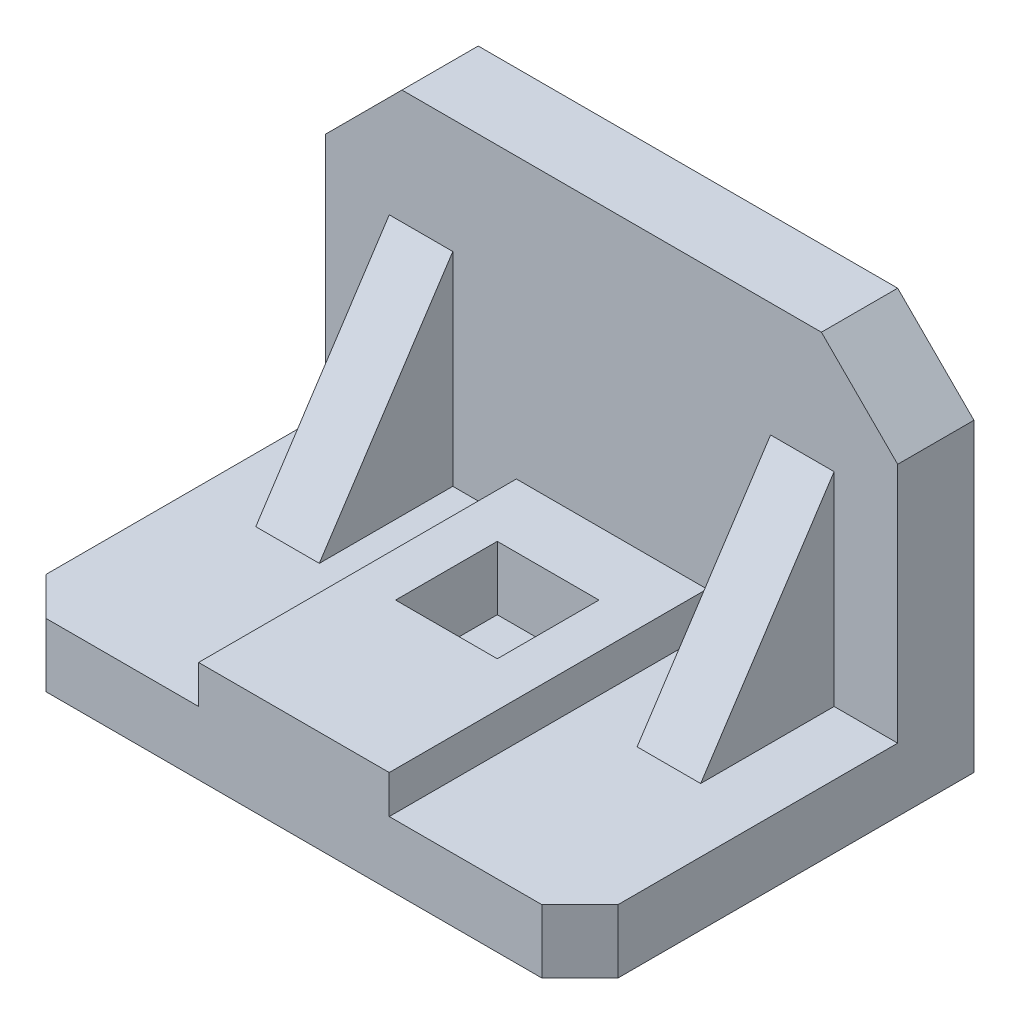
ISO-10303-21;
HEADER;
FILE_DESCRIPTION(('STEP AP214'),'2;1');
FILE_NAME('part.step','',(''),(''),'','','');
FILE_SCHEMA(('AUTOMOTIVE_DESIGN { 1 0 10303 214 1 1 1 1 }'));
ENDSEC;
DATA;
#1=APPLICATION_CONTEXT('core data for automotive mechanical design processes');
#2=APPLICATION_PROTOCOL_DEFINITION('international standard','automotive_design',2000,#1);
#3=PRODUCT_CONTEXT('',#1,'mechanical');
#4=PRODUCT('Part','Part','',(#3));
#5=PRODUCT_RELATED_PRODUCT_CATEGORY('part','',(#4));
#6=PRODUCT_DEFINITION_FORMATION('','',#4);
#7=PRODUCT_DEFINITION_CONTEXT('part definition',#1,'design');
#8=PRODUCT_DEFINITION('design','',#6,#7);
#9=PRODUCT_DEFINITION_SHAPE('','',#8);
#10=(LENGTH_UNIT() NAMED_UNIT(*) SI_UNIT(.MILLI.,.METRE.));
#11=(NAMED_UNIT(*) PLANE_ANGLE_UNIT() SI_UNIT($,.RADIAN.));
#12=(NAMED_UNIT(*) SI_UNIT($,.STERADIAN.) SOLID_ANGLE_UNIT());
#13=UNCERTAINTY_MEASURE_WITH_UNIT(LENGTH_MEASURE(1.E-05),#10,'distance_accuracy_value','');
#14=(GEOMETRIC_REPRESENTATION_CONTEXT(3) GLOBAL_UNCERTAINTY_ASSIGNED_CONTEXT((#13)) GLOBAL_UNIT_ASSIGNED_CONTEXT((#10,
#11,#12)) REPRESENTATION_CONTEXT('',''));
#15=CARTESIAN_POINT('',(0.,0.,0.));
#16=DIRECTION('',(0.,0.,1.));
#17=DIRECTION('',(1.,0.,0.));
#18=AXIS2_PLACEMENT_3D('',#15,#16,#17);
#19=CARTESIAN_POINT('',(73.5797101449275,42.,12.));
#20=DIRECTION('',(0.,0.548656441486822,0.836047910837063));
#21=DIRECTION('',(0.,-0.836047910837063,0.548656441486822));
#22=AXIS2_PLACEMENT_3D('',#19,#20,#21);
#23=PLANE('',#22);
#24=DIRECTION('',(1.,0.,0.));
#25=VECTOR('',#24,1.);
#26=CARTESIAN_POINT('',(73.5797101449275,9.99999999999999,33.));
#27=LINE('',#26,#25);
#28=CARTESIAN_POINT('',(73.5797101449275,10.,33.));
#29=VERTEX_POINT('',#28);
#30=CARTESIAN_POINT('',(83.5797101449275,10.,33.));
#31=VERTEX_POINT('',#30);
#32=EDGE_CURVE('E214',#29,#31,#27,.T.);
#33=ORIENTED_EDGE('',*,*,#32,.T.);
#34=DIRECTION('',(0.,-0.836047910837063,0.548656441486822));
#35=VECTOR('',#34,1.);
#36=CARTESIAN_POINT('',(83.5797101449275,10.,33.));
#37=LINE('',#36,#35);
#38=CARTESIAN_POINT('',(83.5797101449275,42.,12.));
#39=VERTEX_POINT('',#38);
#40=EDGE_CURVE('E217',#39,#31,#37,.T.);
#41=ORIENTED_EDGE('',*,*,#40,.F.);
#42=DIRECTION('',(1.,0.,0.));
#43=VECTOR('',#42,1.);
#44=CARTESIAN_POINT('',(73.5797101449275,42.,12.));
#45=LINE('',#44,#43);
#46=CARTESIAN_POINT('',(73.5797101449275,42.,12.));
#47=VERTEX_POINT('',#46);
#48=EDGE_CURVE('E228',#47,#39,#45,.T.);
#49=ORIENTED_EDGE('',*,*,#48,.F.);
#50=DIRECTION('',(0.,-0.836047910837063,0.548656441486822));
#51=VECTOR('',#50,1.);
#52=CARTESIAN_POINT('',(73.5797101449275,42.,12.));
#53=LINE('',#52,#51);
#54=EDGE_CURVE('E223',#47,#29,#53,.T.);
#55=ORIENTED_EDGE('',*,*,#54,.T.);
#56=EDGE_LOOP('',(#33,#41,#49,#55));
#57=FACE_BOUND('',#56,.T.);
#58=ADVANCED_FACE('F50',(#57),#23,.T.);
#59=CARTESIAN_POINT('',(0.,0.,12.));
#60=DIRECTION('',(0.,0.,1.));
#61=DIRECTION('',(1.,0.,0.));
#62=AXIS2_PLACEMENT_3D('',#59,#60,#61);
#63=PLANE('',#62);
#64=ORIENTED_EDGE('',*,*,#48,.T.);
#65=DIRECTION('',(0.,1.,0.));
#66=VECTOR('',#65,1.);
#67=CARTESIAN_POINT('',(83.5797101449275,42.,12.));
#68=LINE('',#67,#66);
#69=CARTESIAN_POINT('',(83.5797101449275,10.,12.));
#70=VERTEX_POINT('',#69);
#71=EDGE_CURVE('E65',#70,#39,#68,.T.);
#72=ORIENTED_EDGE('',*,*,#71,.F.);
#73=DIRECTION('',(1.,0.,0.));
#74=VECTOR('',#73,1.);
#75=CARTESIAN_POINT('',(83.5797101449275,10.,12.));
#76=LINE('',#75,#74);
#77=CARTESIAN_POINT('',(93.5797101449275,10.,12.));
#78=VERTEX_POINT('',#77);
#79=EDGE_CURVE('E216',#70,#78,#76,.T.);
#80=ORIENTED_EDGE('',*,*,#79,.T.);
#81=DIRECTION('',(0.,1.,0.));
#82=VECTOR('',#81,1.);
#83=CARTESIAN_POINT('',(93.5797101449275,0.,12.));
#84=LINE('',#83,#82);
#85=CARTESIAN_POINT('',(93.5797101449275,48.,12.));
#86=VERTEX_POINT('',#85);
#87=EDGE_CURVE('E362',#78,#86,#84,.T.);
#88=ORIENTED_EDGE('',*,*,#87,.T.);
#89=DIRECTION('',(0.707106781186548,-0.707106781186548,0.));
#90=VECTOR('',#89,1.);
#91=CARTESIAN_POINT('',(70.7898550724637,70.7898550724637,12.));
#92=LINE('',#91,#90);
#93=CARTESIAN_POINT('',(81.5797101449275,60.,12.));
#94=VERTEX_POINT('',#93);
#95=EDGE_CURVE('E352',#94,#86,#92,.T.);
#96=ORIENTED_EDGE('',*,*,#95,.F.);
#97=DIRECTION('',(-1.,0.,0.));
#98=VECTOR('',#97,1.);
#99=CARTESIAN_POINT('',(0.,60.,12.));
#100=LINE('',#99,#98);
#101=CARTESIAN_POINT('',(15.5797101449275,60.,12.));
#102=VERTEX_POINT('',#101);
#103=EDGE_CURVE('E358',#94,#102,#100,.T.);
#104=ORIENTED_EDGE('',*,*,#103,.T.);
#105=DIRECTION('',(0.707106781186547,0.707106781186548,0.));
#106=VECTOR('',#105,1.);
#107=CARTESIAN_POINT('',(-22.2101449275362,22.2101449275362,12.));
#108=LINE('',#107,#106);
#109=CARTESIAN_POINT('',(3.57971014492751,48.,12.));
#110=VERTEX_POINT('',#109);
#111=EDGE_CURVE('E360',#110,#102,#108,.T.);
#112=ORIENTED_EDGE('',*,*,#111,.F.);
#113=DIRECTION('',(0.,-1.,0.));
#114=VECTOR('',#113,1.);
#115=CARTESIAN_POINT('',(3.57971014492751,0.,12.));
#116=LINE('',#115,#114);
#117=CARTESIAN_POINT('',(3.57971014492751,9.99999999999999,12.));
#118=VERTEX_POINT('',#117);
#119=EDGE_CURVE('E365',#110,#118,#116,.T.);
#120=ORIENTED_EDGE('',*,*,#119,.T.);
#121=DIRECTION('',(-1.,0.,0.));
#122=VECTOR('',#121,1.);
#123=CARTESIAN_POINT('',(13.5797101449275,9.99999999999999,12.));
#124=LINE('',#123,#122);
#125=CARTESIAN_POINT('',(13.5797101449275,9.99999999999999,12.));
#126=VERTEX_POINT('',#125);
#127=EDGE_CURVE('E237',#126,#118,#124,.T.);
#128=ORIENTED_EDGE('',*,*,#127,.F.);
#129=DIRECTION('',(0.,-1.,0.));
#130=VECTOR('',#129,1.);
#131=CARTESIAN_POINT('',(13.5797101449275,42.,12.));
#132=LINE('',#131,#130);
#133=CARTESIAN_POINT('',(13.5797101449275,42.,12.));
#134=VERTEX_POINT('',#133);
#135=EDGE_CURVE('E230',#134,#126,#132,.T.);
#136=ORIENTED_EDGE('',*,*,#135,.F.);
#137=DIRECTION('',(-1.,0.,0.));
#138=VECTOR('',#137,1.);
#139=CARTESIAN_POINT('',(23.5797101449275,42.,12.));
#140=LINE('',#139,#138);
#141=CARTESIAN_POINT('',(23.5797101449275,42.,12.));
#142=VERTEX_POINT('',#141);
#143=EDGE_CURVE('E249',#142,#134,#140,.T.);
#144=ORIENTED_EDGE('',*,*,#143,.F.);
#145=DIRECTION('',(0.,-1.,0.));
#146=VECTOR('',#145,1.);
#147=CARTESIAN_POINT('',(23.5797101449275,10.,12.));
#148=LINE('',#147,#146);
#149=CARTESIAN_POINT('',(23.5797101449275,10.,12.));
#150=VERTEX_POINT('',#149);
#151=EDGE_CURVE('E250',#142,#150,#148,.T.);
#152=ORIENTED_EDGE('',*,*,#151,.T.);
#153=DIRECTION('',(1.,0.,0.));
#154=VECTOR('',#153,1.);
#155=CARTESIAN_POINT('',(3.57971014492751,10.,12.));
#156=LINE('',#155,#154);
#157=CARTESIAN_POINT('',(33.5797101449275,10.,12.));
#158=VERTEX_POINT('',#157);
#159=EDGE_CURVE('E320',#150,#158,#156,.T.);
#160=ORIENTED_EDGE('',*,*,#159,.T.);
#161=DIRECTION('',(0.,-1.,0.));
#162=VECTOR('',#161,1.);
#163=CARTESIAN_POINT('',(33.5797101449275,16.,12.));
#164=LINE('',#163,#162);
#165=CARTESIAN_POINT('',(33.5797101449275,16.,12.));
#166=VERTEX_POINT('',#165);
#167=EDGE_CURVE('E297',#166,#158,#164,.T.);
#168=ORIENTED_EDGE('',*,*,#167,.F.);
#169=DIRECTION('',(-1.,0.,0.));
#170=VECTOR('',#169,1.);
#171=CARTESIAN_POINT('',(33.5797101449275,16.,12.));
#172=LINE('',#171,#170);
#173=CARTESIAN_POINT('',(63.5797101449275,16.,12.));
#174=VERTEX_POINT('',#173);
#175=EDGE_CURVE('E300',#174,#166,#172,.T.);
#176=ORIENTED_EDGE('',*,*,#175,.F.);
#177=DIRECTION('',(0.,-1.,0.));
#178=VECTOR('',#177,1.);
#179=CARTESIAN_POINT('',(63.5797101449275,16.,12.));
#180=LINE('',#179,#178);
#181=CARTESIAN_POINT('',(63.5797101449275,10.,12.));
#182=VERTEX_POINT('',#181);
#183=EDGE_CURVE('E310',#174,#182,#180,.T.);
#184=ORIENTED_EDGE('',*,*,#183,.T.);
#185=CARTESIAN_POINT('',(73.5797101449275,10.,12.));
#186=VERTEX_POINT('',#185);
#187=EDGE_CURVE('E318',#182,#186,#156,.T.);
#188=ORIENTED_EDGE('',*,*,#187,.T.);
#189=DIRECTION('',(0.,1.,0.));
#190=VECTOR('',#189,1.);
#191=CARTESIAN_POINT('',(73.5797101449275,10.,12.));
#192=LINE('',#191,#190);
#193=EDGE_CURVE('E70',#186,#47,#192,.T.);
#194=ORIENTED_EDGE('',*,*,#193,.T.);
#195=EDGE_LOOP('',(#64,#72,#80,#88,#96,#104,#112,#120,#128,#136,#144,#152,#160,#168,#176,#184,
#188,#194));
#196=FACE_BOUND('',#195,.T.);
#197=ADVANCED_FACE('F417',(#196),#63,.T.);
#198=CARTESIAN_POINT('',(0.,10.,0.));
#199=DIRECTION('',(0.,-1.,0.));
#200=DIRECTION('',(0.,0.,-1.));
#201=AXIS2_PLACEMENT_3D('',#198,#199,#200);
#202=PLANE('',#201);
#203=DIRECTION('',(0.,0.,1.));
#204=VECTOR('',#203,1.);
#205=CARTESIAN_POINT('',(23.5797101449275,10.,12.));
#206=LINE('',#205,#204);
#207=CARTESIAN_POINT('',(23.5797101449275,10.,33.));
#208=VERTEX_POINT('',#207);
#209=EDGE_CURVE('E245',#150,#208,#206,.T.);
#210=ORIENTED_EDGE('',*,*,#209,.T.);
#211=DIRECTION('',(-1.,0.,0.));
#212=VECTOR('',#211,1.);
#213=CARTESIAN_POINT('',(23.5797101449275,10.,33.));
#214=LINE('',#213,#212);
#215=CARTESIAN_POINT('',(13.5797101449275,10.,33.));
#216=VERTEX_POINT('',#215);
#217=EDGE_CURVE('E248',#208,#216,#214,.T.);
#218=ORIENTED_EDGE('',*,*,#217,.T.);
#219=DIRECTION('',(0.,0.,1.));
#220=VECTOR('',#219,1.);
#221=CARTESIAN_POINT('',(13.5797101449275,9.99999999999999,12.));
#222=LINE('',#221,#220);
#223=EDGE_CURVE('E240',#126,#216,#222,.T.);
#224=ORIENTED_EDGE('',*,*,#223,.F.);
#225=ORIENTED_EDGE('',*,*,#127,.T.);
#226=DIRECTION('',(0.,0.,-1.));
#227=VECTOR('',#226,1.);
#228=CARTESIAN_POINT('',(3.57971014492751,10.,12.));
#229=LINE('',#228,#227);
#230=CARTESIAN_POINT('',(3.57971014492751,10.,56.));
#231=VERTEX_POINT('',#230);
#232=EDGE_CURVE('E335',#231,#118,#229,.T.);
#233=ORIENTED_EDGE('',*,*,#232,.F.);
#234=DIRECTION('',(-0.707106781186546,0.,-0.707106781186549));
#235=VECTOR('',#234,1.);
#236=CARTESIAN_POINT('',(3.57971014492751,10.,56.));
#237=LINE('',#236,#235);
#238=CARTESIAN_POINT('',(9.57971014492751,10.,62.));
#239=VERTEX_POINT('',#238);
#240=EDGE_CURVE('E328',#239,#231,#237,.T.);
#241=ORIENTED_EDGE('',*,*,#240,.F.);
#242=DIRECTION('',(-1.,0.,0.));
#243=VECTOR('',#242,1.);
#244=CARTESIAN_POINT('',(87.5797101449275,10.,62.));
#245=LINE('',#244,#243);
#246=CARTESIAN_POINT('',(33.5797101449275,10.,62.));
#247=VERTEX_POINT('',#246);
#248=EDGE_CURVE('E323',#247,#239,#245,.T.);
#249=ORIENTED_EDGE('',*,*,#248,.F.);
#250=DIRECTION('',(0.,0.,1.));
#251=VECTOR('',#250,1.);
#252=CARTESIAN_POINT('',(33.5797101449275,10.,12.));
#253=LINE('',#252,#251);
#254=EDGE_CURVE('E281',#158,#247,#253,.T.);
#255=ORIENTED_EDGE('',*,*,#254,.F.);
#256=ORIENTED_EDGE('',*,*,#159,.F.);
#257=EDGE_LOOP('',(#210,#218,#224,#225,#233,#241,#249,#255,#256));
#258=FACE_BOUND('',#257,.T.);
#259=ADVANCED_FACE('F419',(#258),#202,.F.);
#260=DIRECTION('',(0.,0.,1.));
#261=VECTOR('',#260,1.);
#262=CARTESIAN_POINT('',(93.5797101449275,10.,12.));
#263=LINE('',#262,#261);
#264=CARTESIAN_POINT('',(93.5797101449275,10.,56.));
#265=VERTEX_POINT('',#264);
#266=EDGE_CURVE('E316',#78,#265,#263,.T.);
#267=ORIENTED_EDGE('',*,*,#266,.F.);
#268=ORIENTED_EDGE('',*,*,#79,.F.);
#269=DIRECTION('',(0.,0.,-1.));
#270=VECTOR('',#269,1.);
#271=CARTESIAN_POINT('',(83.5797101449275,10.,12.));
#272=LINE('',#271,#270);
#273=EDGE_CURVE('E209',#31,#70,#272,.T.);
#274=ORIENTED_EDGE('',*,*,#273,.F.);
#275=ORIENTED_EDGE('',*,*,#32,.F.);
#276=DIRECTION('',(0.,0.,-1.));
#277=VECTOR('',#276,1.);
#278=CARTESIAN_POINT('',(73.5797101449275,9.99999999999999,33.));
#279=LINE('',#278,#277);
#280=EDGE_CURVE('E771',#29,#186,#279,.T.);
#281=ORIENTED_EDGE('',*,*,#280,.T.);
#282=ORIENTED_EDGE('',*,*,#187,.F.);
#283=DIRECTION('',(0.,0.,-1.));
#284=VECTOR('',#283,1.);
#285=CARTESIAN_POINT('',(63.5797101449275,10.,12.));
#286=LINE('',#285,#284);
#287=CARTESIAN_POINT('',(63.5797101449275,10.,62.));
#288=VERTEX_POINT('',#287);
#289=EDGE_CURVE('E292',#288,#182,#286,.T.);
#290=ORIENTED_EDGE('',*,*,#289,.F.);
#291=CARTESIAN_POINT('',(87.5797101449275,10.,62.));
#292=VERTEX_POINT('',#291);
#293=EDGE_CURVE('E326',#292,#288,#245,.T.);
#294=ORIENTED_EDGE('',*,*,#293,.F.);
#295=DIRECTION('',(-0.707106781186548,0.,0.707106781186547));
#296=VECTOR('',#295,1.);
#297=CARTESIAN_POINT('',(87.5797101449275,10.,62.));
#298=LINE('',#297,#296);
#299=EDGE_CURVE('E325',#265,#292,#298,.T.);
#300=ORIENTED_EDGE('',*,*,#299,.F.);
#301=EDGE_LOOP('',(#267,#268,#274,#275,#281,#282,#290,#294,#300));
#302=FACE_BOUND('',#301,.T.);
#303=ADVANCED_FACE('F212',(#302),#202,.F.);
#304=CARTESIAN_POINT('',(70.7898550724637,70.7898550724637,12.));
#305=DIRECTION('',(0.707106781186547,0.707106781186547,0.));
#306=DIRECTION('',(-0.707106781186548,0.707106781186548,0.));
#307=AXIS2_PLACEMENT_3D('',#304,#305,#306);
#308=PLANE('',#307);
#309=DIRECTION('',(0.707106781186548,-0.707106781186548,0.));
#310=VECTOR('',#309,1.);
#311=CARTESIAN_POINT('',(70.7898550724637,70.7898550724637,0.));
#312=LINE('',#311,#310);
#313=CARTESIAN_POINT('',(81.5797101449275,60.,0.));
#314=VERTEX_POINT('',#313);
#315=CARTESIAN_POINT('',(93.5797101449275,48.,0.));
#316=VERTEX_POINT('',#315);
#317=EDGE_CURVE('E346',#314,#316,#312,.T.);
#318=ORIENTED_EDGE('',*,*,#317,.F.);
#319=DIRECTION('',(0.,0.,-1.));
#320=VECTOR('',#319,1.);
#321=CARTESIAN_POINT('',(81.5797101449275,60.,12.));
#322=LINE('',#321,#320);
#323=EDGE_CURVE('E11',#94,#314,#322,.T.);
#324=ORIENTED_EDGE('',*,*,#323,.F.);
#325=ORIENTED_EDGE('',*,*,#95,.T.);
#326=DIRECTION('',(0.,0.,-1.));
#327=VECTOR('',#326,1.);
#328=CARTESIAN_POINT('',(93.5797101449275,48.,12.));
#329=LINE('',#328,#327);
#330=EDGE_CURVE('E370',#86,#316,#329,.T.);
#331=ORIENTED_EDGE('',*,*,#330,.T.);
#332=EDGE_LOOP('',(#318,#324,#325,#331));
#333=FACE_BOUND('',#332,.T.);
#334=ADVANCED_FACE('F47',(#333),#308,.T.);
#335=CARTESIAN_POINT('',(0.,60.,12.));
#336=DIRECTION('',(0.,-1.,0.));
#337=DIRECTION('',(1.,0.,0.));
#338=AXIS2_PLACEMENT_3D('',#335,#336,#337);
#339=PLANE('',#338);
#340=DIRECTION('',(-1.,0.,0.));
#341=VECTOR('',#340,1.);
#342=CARTESIAN_POINT('',(0.,60.,0.));
#343=LINE('',#342,#341);
#344=CARTESIAN_POINT('',(15.5797101449275,60.,0.));
#345=VERTEX_POINT('',#344);
#346=EDGE_CURVE('E369',#314,#345,#343,.T.);
#347=ORIENTED_EDGE('',*,*,#346,.T.);
#348=DIRECTION('',(0.,0.,-1.));
#349=VECTOR('',#348,1.);
#350=CARTESIAN_POINT('',(15.5797101449275,60.,12.));
#351=LINE('',#350,#349);
#352=EDGE_CURVE('E54',#102,#345,#351,.T.);
#353=ORIENTED_EDGE('',*,*,#352,.F.);
#354=ORIENTED_EDGE('',*,*,#103,.F.);
#355=ORIENTED_EDGE('',*,*,#323,.T.);
#356=EDGE_LOOP('',(#347,#353,#354,#355));
#357=FACE_BOUND('',#356,.T.);
#358=ADVANCED_FACE('F397',(#357),#339,.F.);
#359=CARTESIAN_POINT('',(-22.2101449275362,22.2101449275362,12.));
#360=DIRECTION('',(-0.707106781186548,0.707106781186547,0.));
#361=DIRECTION('',(-0.707106781186547,-0.707106781186548,0.));
#362=AXIS2_PLACEMENT_3D('',#359,#360,#361);
#363=PLANE('',#362);
#364=DIRECTION('',(0.707106781186547,0.707106781186548,0.));
#365=VECTOR('',#364,1.);
#366=CARTESIAN_POINT('',(-22.2101449275362,22.2101449275362,0.));
#367=LINE('',#366,#365);
#368=CARTESIAN_POINT('',(3.57971014492751,48.,0.));
#369=VERTEX_POINT('',#368);
#370=EDGE_CURVE('E373',#369,#345,#367,.T.);
#371=ORIENTED_EDGE('',*,*,#370,.F.);
#372=DIRECTION('',(0.,0.,-1.));
#373=VECTOR('',#372,1.);
#374=CARTESIAN_POINT('',(3.57971014492751,48.,12.));
#375=LINE('',#374,#373);
#376=EDGE_CURVE('E386',#110,#369,#375,.T.);
#377=ORIENTED_EDGE('',*,*,#376,.F.);
#378=ORIENTED_EDGE('',*,*,#111,.T.);
#379=ORIENTED_EDGE('',*,*,#352,.T.);
#380=EDGE_LOOP('',(#371,#377,#378,#379));
#381=FACE_BOUND('',#380,.T.);
#382=ADVANCED_FACE('F394',(#381),#363,.T.);
#383=CARTESIAN_POINT('',(3.57971014492751,0.,12.));
#384=DIRECTION('',(1.,0.,0.));
#385=DIRECTION('',(0.,1.,0.));
#386=AXIS2_PLACEMENT_3D('',#383,#384,#385);
#387=PLANE('',#386);
#388=ORIENTED_EDGE('',*,*,#232,.T.);
#389=ORIENTED_EDGE('',*,*,#119,.F.);
#390=ORIENTED_EDGE('',*,*,#376,.T.);
#391=DIRECTION('',(0.,-1.,0.));
#392=VECTOR('',#391,1.);
#393=CARTESIAN_POINT('',(3.57971014492751,0.,0.));
#394=LINE('',#393,#392);
#395=CARTESIAN_POINT('',(3.57971014492751,0.,0.));
#396=VERTEX_POINT('',#395);
#397=EDGE_CURVE('E376',#369,#396,#394,.T.);
#398=ORIENTED_EDGE('',*,*,#397,.T.);
#399=DIRECTION('',(0.,0.,-1.));
#400=VECTOR('',#399,1.);
#401=CARTESIAN_POINT('',(3.57971014492751,0.,12.));
#402=LINE('',#401,#400);
#403=CARTESIAN_POINT('',(3.57971014492751,0.,56.));
#404=VERTEX_POINT('',#403);
#405=EDGE_CURVE('E387',#404,#396,#402,.T.);
#406=ORIENTED_EDGE('',*,*,#405,.F.);
#407=DIRECTION('',(0.,-1.,0.));
#408=VECTOR('',#407,1.);
#409=CARTESIAN_POINT('',(3.57971014492751,10.,56.));
#410=LINE('',#409,#408);
#411=EDGE_CURVE('E344',#231,#404,#410,.T.);
#412=ORIENTED_EDGE('',*,*,#411,.F.);
#413=EDGE_LOOP('',(#388,#389,#390,#398,#406,#412));
#414=FACE_BOUND('',#413,.T.);
#415=ADVANCED_FACE('F407',(#414),#387,.F.);
#416=CARTESIAN_POINT('',(0.,0.,12.));
#417=DIRECTION('',(0.,1.,0.));
#418=DIRECTION('',(0.,0.,1.));
#419=AXIS2_PLACEMENT_3D('',#416,#417,#418);
#420=PLANE('',#419);
#421=DIRECTION('',(1.,0.,0.));
#422=VECTOR('',#421,1.);
#423=CARTESIAN_POINT('',(0.,0.,0.));
#424=LINE('',#423,#422);
#425=CARTESIAN_POINT('',(93.5797101449275,0.,0.));
#426=VERTEX_POINT('',#425);
#427=EDGE_CURVE('E377',#396,#426,#424,.T.);
#428=ORIENTED_EDGE('',*,*,#427,.T.);
#429=DIRECTION('',(0.,0.,-1.));
#430=VECTOR('',#429,1.);
#431=CARTESIAN_POINT('',(93.5797101449275,0.,12.));
#432=LINE('',#431,#430);
#433=CARTESIAN_POINT('',(93.5797101449275,0.,56.));
#434=VERTEX_POINT('',#433);
#435=EDGE_CURVE('E384',#434,#426,#432,.T.);
#436=ORIENTED_EDGE('',*,*,#435,.F.);
#437=DIRECTION('',(-0.707106781186548,0.,0.707106781186547));
#438=VECTOR('',#437,1.);
#439=CARTESIAN_POINT('',(87.5797101449275,0.,62.));
#440=LINE('',#439,#438);
#441=CARTESIAN_POINT('',(87.5797101449275,0.,62.));
#442=VERTEX_POINT('',#441);
#443=EDGE_CURVE('E317',#434,#442,#440,.T.);
#444=ORIENTED_EDGE('',*,*,#443,.T.);
#445=DIRECTION('',(-1.,0.,0.));
#446=VECTOR('',#445,1.);
#447=CARTESIAN_POINT('',(87.5797101449275,0.,62.));
#448=LINE('',#447,#446);
#449=CARTESIAN_POINT('',(9.57971014492751,0.,62.));
#450=VERTEX_POINT('',#449);
#451=EDGE_CURVE('E340',#442,#450,#448,.T.);
#452=ORIENTED_EDGE('',*,*,#451,.T.);
#453=DIRECTION('',(-0.707106781186546,0.,-0.707106781186549));
#454=VECTOR('',#453,1.);
#455=CARTESIAN_POINT('',(3.57971014492751,0.,56.));
#456=LINE('',#455,#454);
#457=EDGE_CURVE('E338',#450,#404,#456,.T.);
#458=ORIENTED_EDGE('',*,*,#457,.T.);
#459=ORIENTED_EDGE('',*,*,#405,.T.);
#460=EDGE_LOOP('',(#428,#436,#444,#452,#458,#459));
#461=FACE_BOUND('',#460,.T.);
#462=ADVANCED_FACE('F406',(#461),#420,.F.);
#463=CARTESIAN_POINT('',(93.5797101449275,0.,12.));
#464=DIRECTION('',(-1.,0.,0.));
#465=DIRECTION('',(0.,-1.,0.));
#466=AXIS2_PLACEMENT_3D('',#463,#464,#465);
#467=PLANE('',#466);
#468=ORIENTED_EDGE('',*,*,#87,.F.);
#469=ORIENTED_EDGE('',*,*,#266,.T.);
#470=DIRECTION('',(0.,-1.,0.));
#471=VECTOR('',#470,1.);
#472=CARTESIAN_POINT('',(93.5797101449275,10.,56.));
#473=LINE('',#472,#471);
#474=EDGE_CURVE('E333',#265,#434,#473,.T.);
#475=ORIENTED_EDGE('',*,*,#474,.T.);
#476=ORIENTED_EDGE('',*,*,#435,.T.);
#477=DIRECTION('',(0.,1.,0.));
#478=VECTOR('',#477,1.);
#479=CARTESIAN_POINT('',(93.5797101449275,0.,0.));
#480=LINE('',#479,#478);
#481=EDGE_CURVE('E357',#426,#316,#480,.T.);
#482=ORIENTED_EDGE('',*,*,#481,.T.);
#483=ORIENTED_EDGE('',*,*,#330,.F.);
#484=EDGE_LOOP('',(#468,#469,#475,#476,#482,#483));
#485=FACE_BOUND('',#484,.T.);
#486=ADVANCED_FACE('F586',(#485),#467,.F.);
#487=CARTESIAN_POINT('',(0.,0.,0.));
#488=DIRECTION('',(0.,0.,1.));
#489=DIRECTION('',(1.,0.,0.));
#490=AXIS2_PLACEMENT_3D('',#487,#488,#489);
#491=PLANE('',#490);
#492=ORIENTED_EDGE('',*,*,#317,.T.);
#493=ORIENTED_EDGE('',*,*,#481,.F.);
#494=ORIENTED_EDGE('',*,*,#427,.F.);
#495=ORIENTED_EDGE('',*,*,#397,.F.);
#496=ORIENTED_EDGE('',*,*,#370,.T.);
#497=ORIENTED_EDGE('',*,*,#346,.F.);
#498=EDGE_LOOP('',(#492,#493,#494,#495,#496,#497));
#499=FACE_BOUND('',#498,.T.);
#500=ADVANCED_FACE('F405',(#499),#491,.F.);
#501=CARTESIAN_POINT('',(3.57971014492751,10.,56.));
#502=DIRECTION('',(-0.707106781186549,0.,0.707106781186546));
#503=DIRECTION('',(0.707106781186546,0.,0.707106781186549));
#504=AXIS2_PLACEMENT_3D('',#501,#502,#503);
#505=PLANE('',#504);
#506=ORIENTED_EDGE('',*,*,#457,.F.);
#507=DIRECTION('',(0.,-1.,0.));
#508=VECTOR('',#507,1.);
#509=CARTESIAN_POINT('',(9.57971014492751,10.,62.));
#510=LINE('',#509,#508);
#511=EDGE_CURVE('E347',#239,#450,#510,.T.);
#512=ORIENTED_EDGE('',*,*,#511,.F.);
#513=ORIENTED_EDGE('',*,*,#240,.T.);
#514=ORIENTED_EDGE('',*,*,#411,.T.);
#515=EDGE_LOOP('',(#506,#512,#513,#514));
#516=FACE_BOUND('',#515,.T.);
#517=ADVANCED_FACE('F413',(#516),#505,.T.);
#518=CARTESIAN_POINT('',(87.5797101449275,10.,62.));
#519=DIRECTION('',(0.,0.,1.));
#520=DIRECTION('',(1.,0.,0.));
#521=AXIS2_PLACEMENT_3D('',#518,#519,#520);
#522=PLANE('',#521);
#523=ORIENTED_EDGE('',*,*,#451,.F.);
#524=DIRECTION('',(0.,-1.,0.));
#525=VECTOR('',#524,1.);
#526=CARTESIAN_POINT('',(87.5797101449275,10.,62.));
#527=LINE('',#526,#525);
#528=EDGE_CURVE('E348',#292,#442,#527,.T.);
#529=ORIENTED_EDGE('',*,*,#528,.F.);
#530=ORIENTED_EDGE('',*,*,#293,.T.);
#531=DIRECTION('',(0.,-1.,0.));
#532=VECTOR('',#531,1.);
#533=CARTESIAN_POINT('',(63.5797101449275,16.,62.));
#534=LINE('',#533,#532);
#535=CARTESIAN_POINT('',(63.5797101449275,16.,62.));
#536=VERTEX_POINT('',#535);
#537=EDGE_CURVE('E309',#536,#288,#534,.T.);
#538=ORIENTED_EDGE('',*,*,#537,.F.);
#539=DIRECTION('',(1.,0.,0.));
#540=VECTOR('',#539,1.);
#541=CARTESIAN_POINT('',(33.5797101449275,16.,62.));
#542=LINE('',#541,#540);
#543=CARTESIAN_POINT('',(33.5797101449275,16.,62.));
#544=VERTEX_POINT('',#543);
#545=EDGE_CURVE('E293',#544,#536,#542,.T.);
#546=ORIENTED_EDGE('',*,*,#545,.F.);
#547=DIRECTION('',(0.,-1.,0.));
#548=VECTOR('',#547,1.);
#549=CARTESIAN_POINT('',(33.5797101449275,16.,62.));
#550=LINE('',#549,#548);
#551=EDGE_CURVE('E312',#544,#247,#550,.T.);
#552=ORIENTED_EDGE('',*,*,#551,.T.);
#553=ORIENTED_EDGE('',*,*,#248,.T.);
#554=ORIENTED_EDGE('',*,*,#511,.T.);
#555=EDGE_LOOP('',(#523,#529,#530,#538,#546,#552,#553,#554));
#556=FACE_BOUND('',#555,.T.);
#557=ADVANCED_FACE('F678',(#556),#522,.T.);
#558=CARTESIAN_POINT('',(87.5797101449275,10.,62.));
#559=DIRECTION('',(0.707106781186547,0.,0.707106781186548));
#560=DIRECTION('',(0.707106781186548,0.,-0.707106781186547));
#561=AXIS2_PLACEMENT_3D('',#558,#559,#560);
#562=PLANE('',#561);
#563=ORIENTED_EDGE('',*,*,#443,.F.);
#564=ORIENTED_EDGE('',*,*,#474,.F.);
#565=ORIENTED_EDGE('',*,*,#299,.T.);
#566=ORIENTED_EDGE('',*,*,#528,.T.);
#567=EDGE_LOOP('',(#563,#564,#565,#566));
#568=FACE_BOUND('',#567,.T.);
#569=ADVANCED_FACE('F558',(#568),#562,.T.);
#570=CARTESIAN_POINT('',(33.5797101449275,16.,12.));
#571=DIRECTION('',(1.,0.,0.));
#572=DIRECTION('',(0.,0.,-1.));
#573=AXIS2_PLACEMENT_3D('',#570,#571,#572);
#574=PLANE('',#573);
#575=ORIENTED_EDGE('',*,*,#254,.T.);
#576=ORIENTED_EDGE('',*,*,#551,.F.);
#577=DIRECTION('',(0.,0.,1.));
#578=VECTOR('',#577,1.);
#579=CARTESIAN_POINT('',(33.5797101449275,16.,12.));
#580=LINE('',#579,#578);
#581=EDGE_CURVE('E287',#166,#544,#580,.T.);
#582=ORIENTED_EDGE('',*,*,#581,.F.);
#583=ORIENTED_EDGE('',*,*,#167,.T.);
#584=EDGE_LOOP('',(#575,#576,#582,#583));
#585=FACE_BOUND('',#584,.T.);
#586=ADVANCED_FACE('F548',(#585),#574,.F.);
#587=CARTESIAN_POINT('',(63.5797101449275,16.,12.));
#588=DIRECTION('',(-1.,0.,0.));
#589=DIRECTION('',(0.,0.,1.));
#590=AXIS2_PLACEMENT_3D('',#587,#588,#589);
#591=PLANE('',#590);
#592=ORIENTED_EDGE('',*,*,#289,.T.);
#593=ORIENTED_EDGE('',*,*,#183,.F.);
#594=DIRECTION('',(0.,0.,-1.));
#595=VECTOR('',#594,1.);
#596=CARTESIAN_POINT('',(63.5797101449275,16.,12.));
#597=LINE('',#596,#595);
#598=EDGE_CURVE('E295',#536,#174,#597,.T.);
#599=ORIENTED_EDGE('',*,*,#598,.F.);
#600=ORIENTED_EDGE('',*,*,#537,.T.);
#601=EDGE_LOOP('',(#592,#593,#599,#600));
#602=FACE_BOUND('',#601,.T.);
#603=ADVANCED_FACE('F539',(#602),#591,.F.);
#604=CARTESIAN_POINT('',(0.,16.,0.));
#605=DIRECTION('',(0.,1.,0.));
#606=DIRECTION('',(0.,0.,1.));
#607=AXIS2_PLACEMENT_3D('',#604,#605,#606);
#608=PLANE('',#607);
#609=DIRECTION('',(0.,0.,1.));
#610=VECTOR('',#609,1.);
#611=CARTESIAN_POINT('',(40.5797101449275,16.,22.));
#612=LINE('',#611,#610);
#613=CARTESIAN_POINT('',(40.5797101449275,16.,22.));
#614=VERTEX_POINT('',#613);
#615=CARTESIAN_POINT('',(40.5797101449275,16.,38.));
#616=VERTEX_POINT('',#615);
#617=EDGE_CURVE('E254',#614,#616,#612,.T.);
#618=ORIENTED_EDGE('',*,*,#617,.F.);
#619=DIRECTION('',(-1.,0.,0.));
#620=VECTOR('',#619,1.);
#621=CARTESIAN_POINT('',(40.5797101449275,16.,22.));
#622=LINE('',#621,#620);
#623=CARTESIAN_POINT('',(56.5797101449275,16.,22.));
#624=VERTEX_POINT('',#623);
#625=EDGE_CURVE('E258',#624,#614,#622,.T.);
#626=ORIENTED_EDGE('',*,*,#625,.F.);
#627=DIRECTION('',(0.,0.,-1.));
#628=VECTOR('',#627,1.);
#629=CARTESIAN_POINT('',(56.5797101449275,16.,22.));
#630=LINE('',#629,#628);
#631=CARTESIAN_POINT('',(56.5797101449275,16.,38.));
#632=VERTEX_POINT('',#631);
#633=EDGE_CURVE('E274',#632,#624,#630,.T.);
#634=ORIENTED_EDGE('',*,*,#633,.F.);
#635=DIRECTION('',(1.,0.,0.));
#636=VECTOR('',#635,1.);
#637=CARTESIAN_POINT('',(40.5797101449275,16.,38.));
#638=LINE('',#637,#636);
#639=EDGE_CURVE('E272',#616,#632,#638,.T.);
#640=ORIENTED_EDGE('',*,*,#639,.F.);
#641=EDGE_LOOP('',(#618,#626,#634,#640));
#642=FACE_BOUND('',#641,.T.);
#643=ORIENTED_EDGE('',*,*,#581,.T.);
#644=ORIENTED_EDGE('',*,*,#545,.T.);
#645=ORIENTED_EDGE('',*,*,#598,.T.);
#646=ORIENTED_EDGE('',*,*,#175,.T.);
#647=EDGE_LOOP('',(#643,#644,#645,#646));
#648=FACE_BOUND('',#647,.T.);
#649=ADVANCED_FACE('F530',(#642,#648),#608,.T.);
#650=CARTESIAN_POINT('',(40.5797101449275,6.,22.));
#651=DIRECTION('',(-1.,0.,0.));
#652=DIRECTION('',(0.,0.,1.));
#653=AXIS2_PLACEMENT_3D('',#650,#651,#652);
#654=PLANE('',#653);
#655=ORIENTED_EDGE('',*,*,#617,.T.);
#656=DIRECTION('',(0.,1.,0.));
#657=VECTOR('',#656,1.);
#658=CARTESIAN_POINT('',(40.5797101449275,6.,38.));
#659=LINE('',#658,#657);
#660=CARTESIAN_POINT('',(40.5797101449275,6.,38.));
#661=VERTEX_POINT('',#660);
#662=EDGE_CURVE('E268',#661,#616,#659,.T.);
#663=ORIENTED_EDGE('',*,*,#662,.F.);
#664=DIRECTION('',(0.,0.,1.));
#665=VECTOR('',#664,1.);
#666=CARTESIAN_POINT('',(40.5797101449275,6.,22.));
#667=LINE('',#666,#665);
#668=CARTESIAN_POINT('',(40.5797101449275,6.,22.));
#669=VERTEX_POINT('',#668);
#670=EDGE_CURVE('E257',#669,#661,#667,.T.);
#671=ORIENTED_EDGE('',*,*,#670,.F.);
#672=DIRECTION('',(0.,1.,0.));
#673=VECTOR('',#672,1.);
#674=CARTESIAN_POINT('',(40.5797101449275,6.,22.));
#675=LINE('',#674,#673);
#676=EDGE_CURVE('E276',#669,#614,#675,.T.);
#677=ORIENTED_EDGE('',*,*,#676,.T.);
#678=EDGE_LOOP('',(#655,#663,#671,#677));
#679=FACE_BOUND('',#678,.T.);
#680=ADVANCED_FACE('F520',(#679),#654,.F.);
#681=CARTESIAN_POINT('',(40.5797101449275,6.,22.));
#682=DIRECTION('',(0.,0.,-1.));
#683=DIRECTION('',(-1.,0.,0.));
#684=AXIS2_PLACEMENT_3D('',#681,#682,#683);
#685=PLANE('',#684);
#686=ORIENTED_EDGE('',*,*,#625,.T.);
#687=ORIENTED_EDGE('',*,*,#676,.F.);
#688=DIRECTION('',(-1.,0.,0.));
#689=VECTOR('',#688,1.);
#690=CARTESIAN_POINT('',(40.5797101449275,6.,22.));
#691=LINE('',#690,#689);
#692=CARTESIAN_POINT('',(56.5797101449275,6.,22.));
#693=VERTEX_POINT('',#692);
#694=EDGE_CURVE('E266',#693,#669,#691,.T.);
#695=ORIENTED_EDGE('',*,*,#694,.F.);
#696=DIRECTION('',(0.,1.,0.));
#697=VECTOR('',#696,1.);
#698=CARTESIAN_POINT('',(56.5797101449275,6.,22.));
#699=LINE('',#698,#697);
#700=EDGE_CURVE('E282',#693,#624,#699,.T.);
#701=ORIENTED_EDGE('',*,*,#700,.T.);
#702=EDGE_LOOP('',(#686,#687,#695,#701));
#703=FACE_BOUND('',#702,.T.);
#704=ADVANCED_FACE('F510',(#703),#685,.F.);
#705=CARTESIAN_POINT('',(56.5797101449275,6.,22.));
#706=DIRECTION('',(1.,0.,0.));
#707=DIRECTION('',(0.,0.,-1.));
#708=AXIS2_PLACEMENT_3D('',#705,#706,#707);
#709=PLANE('',#708);
#710=ORIENTED_EDGE('',*,*,#633,.T.);
#711=ORIENTED_EDGE('',*,*,#700,.F.);
#712=DIRECTION('',(0.,0.,-1.));
#713=VECTOR('',#712,1.);
#714=CARTESIAN_POINT('',(56.5797101449275,6.,22.));
#715=LINE('',#714,#713);
#716=CARTESIAN_POINT('',(56.5797101449275,6.,38.));
#717=VERTEX_POINT('',#716);
#718=EDGE_CURVE('E264',#717,#693,#715,.T.);
#719=ORIENTED_EDGE('',*,*,#718,.F.);
#720=DIRECTION('',(0.,1.,0.));
#721=VECTOR('',#720,1.);
#722=CARTESIAN_POINT('',(56.5797101449275,6.,38.));
#723=LINE('',#722,#721);
#724=EDGE_CURVE('E283',#717,#632,#723,.T.);
#725=ORIENTED_EDGE('',*,*,#724,.T.);
#726=EDGE_LOOP('',(#710,#711,#719,#725));
#727=FACE_BOUND('',#726,.T.);
#728=ADVANCED_FACE('F500',(#727),#709,.F.);
#729=CARTESIAN_POINT('',(40.5797101449275,6.,38.));
#730=DIRECTION('',(0.,0.,1.));
#731=DIRECTION('',(1.,0.,0.));
#732=AXIS2_PLACEMENT_3D('',#729,#730,#731);
#733=PLANE('',#732);
#734=ORIENTED_EDGE('',*,*,#639,.T.);
#735=ORIENTED_EDGE('',*,*,#724,.F.);
#736=DIRECTION('',(1.,0.,0.));
#737=VECTOR('',#736,1.);
#738=CARTESIAN_POINT('',(40.5797101449275,6.,38.));
#739=LINE('',#738,#737);
#740=EDGE_CURVE('E256',#661,#717,#739,.T.);
#741=ORIENTED_EDGE('',*,*,#740,.F.);
#742=ORIENTED_EDGE('',*,*,#662,.T.);
#743=EDGE_LOOP('',(#734,#735,#741,#742));
#744=FACE_BOUND('',#743,.T.);
#745=ADVANCED_FACE('F487',(#744),#733,.F.);
#746=CARTESIAN_POINT('',(0.,6.,0.));
#747=DIRECTION('',(0.,1.,0.));
#748=DIRECTION('',(0.,0.,1.));
#749=AXIS2_PLACEMENT_3D('',#746,#747,#748);
#750=PLANE('',#749);
#751=ORIENTED_EDGE('',*,*,#670,.T.);
#752=ORIENTED_EDGE('',*,*,#740,.T.);
#753=ORIENTED_EDGE('',*,*,#718,.T.);
#754=ORIENTED_EDGE('',*,*,#694,.T.);
#755=EDGE_LOOP('',(#751,#752,#753,#754));
#756=FACE_BOUND('',#755,.T.);
#757=ADVANCED_FACE('F445',(#756),#750,.T.);
#758=CARTESIAN_POINT('',(23.5797101449275,10.,33.));
#759=DIRECTION('',(0.,0.548656441486822,0.836047910837063));
#760=DIRECTION('',(0.,-0.836047910837063,0.548656441486822));
#761=AXIS2_PLACEMENT_3D('',#758,#759,#760);
#762=PLANE('',#761);
#763=DIRECTION('',(0.,0.836047910837063,-0.548656441486822));
#764=VECTOR('',#763,1.);
#765=CARTESIAN_POINT('',(13.5797101449275,10.,33.));
#766=LINE('',#765,#764);
#767=EDGE_CURVE('E224',#216,#134,#766,.T.);
#768=ORIENTED_EDGE('',*,*,#767,.F.);
#769=ORIENTED_EDGE('',*,*,#217,.F.);
#770=DIRECTION('',(0.,0.836047910837063,-0.548656441486822));
#771=VECTOR('',#770,1.);
#772=CARTESIAN_POINT('',(23.5797101449275,10.,33.));
#773=LINE('',#772,#771);
#774=EDGE_CURVE('E242',#208,#142,#773,.T.);
#775=ORIENTED_EDGE('',*,*,#774,.T.);
#776=ORIENTED_EDGE('',*,*,#143,.T.);
#777=EDGE_LOOP('',(#768,#769,#775,#776));
#778=FACE_BOUND('',#777,.T.);
#779=ADVANCED_FACE('F428',(#778),#762,.T.);
#780=CARTESIAN_POINT('',(23.5797101449275,0.,0.));
#781=DIRECTION('',(-1.,0.,0.));
#782=DIRECTION('',(0.,-1.,0.));
#783=AXIS2_PLACEMENT_3D('',#780,#781,#782);
#784=PLANE('',#783);
#785=ORIENTED_EDGE('',*,*,#209,.F.);
#786=ORIENTED_EDGE('',*,*,#151,.F.);
#787=ORIENTED_EDGE('',*,*,#774,.F.);
#788=EDGE_LOOP('',(#785,#786,#787));
#789=FACE_BOUND('',#788,.T.);
#790=ADVANCED_FACE('F433',(#789),#784,.F.);
#791=CARTESIAN_POINT('',(13.5797101449275,0.,0.));
#792=DIRECTION('',(1.,0.,0.));
#793=DIRECTION('',(0.,1.,0.));
#794=AXIS2_PLACEMENT_3D('',#791,#792,#793);
#795=PLANE('',#794);
#796=ORIENTED_EDGE('',*,*,#767,.T.);
#797=ORIENTED_EDGE('',*,*,#135,.T.);
#798=ORIENTED_EDGE('',*,*,#223,.T.);
#799=EDGE_LOOP('',(#796,#797,#798));
#800=FACE_BOUND('',#799,.T.);
#801=ADVANCED_FACE('F425',(#800),#795,.F.);
#802=CARTESIAN_POINT('',(73.5797101449275,0.,0.));
#803=DIRECTION('',(1.,0.,0.));
#804=DIRECTION('',(0.,1.,0.));
#805=AXIS2_PLACEMENT_3D('',#802,#803,#804);
#806=PLANE('',#805);
#807=ORIENTED_EDGE('',*,*,#280,.F.);
#808=ORIENTED_EDGE('',*,*,#54,.F.);
#809=ORIENTED_EDGE('',*,*,#193,.F.);
#810=EDGE_LOOP('',(#807,#808,#809));
#811=FACE_BOUND('',#810,.T.);
#812=ADVANCED_FACE('F439',(#811),#806,.F.);
#813=CARTESIAN_POINT('',(83.5797101449275,0.,0.));
#814=DIRECTION('',(1.,0.,0.));
#815=DIRECTION('',(0.,1.,0.));
#816=AXIS2_PLACEMENT_3D('',#813,#814,#815);
#817=PLANE('',#816);
#818=ORIENTED_EDGE('',*,*,#40,.T.);
#819=ORIENTED_EDGE('',*,*,#273,.T.);
#820=ORIENTED_EDGE('',*,*,#71,.T.);
#821=EDGE_LOOP('',(#818,#819,#820));
#822=FACE_BOUND('',#821,.T.);
#823=ADVANCED_FACE('F218',(#822),#817,.T.);
#824=CLOSED_SHELL('',(#58,#197,#259,#303,#334,#358,#382,#415,#462,#486,#500,#517,#557,#569,#586,
#603,#649,#680,#704,#728,#745,#757,#779,#790,#801,#812,#823));
#825=MANIFOLD_SOLID_BREP('B2',#824);
#826=ADVANCED_BREP_SHAPE_REPRESENTATION('',(#18,#825),#14);
#827=SHAPE_DEFINITION_REPRESENTATION(#9,#826);
ENDSEC;
END-ISO-10303-21;
